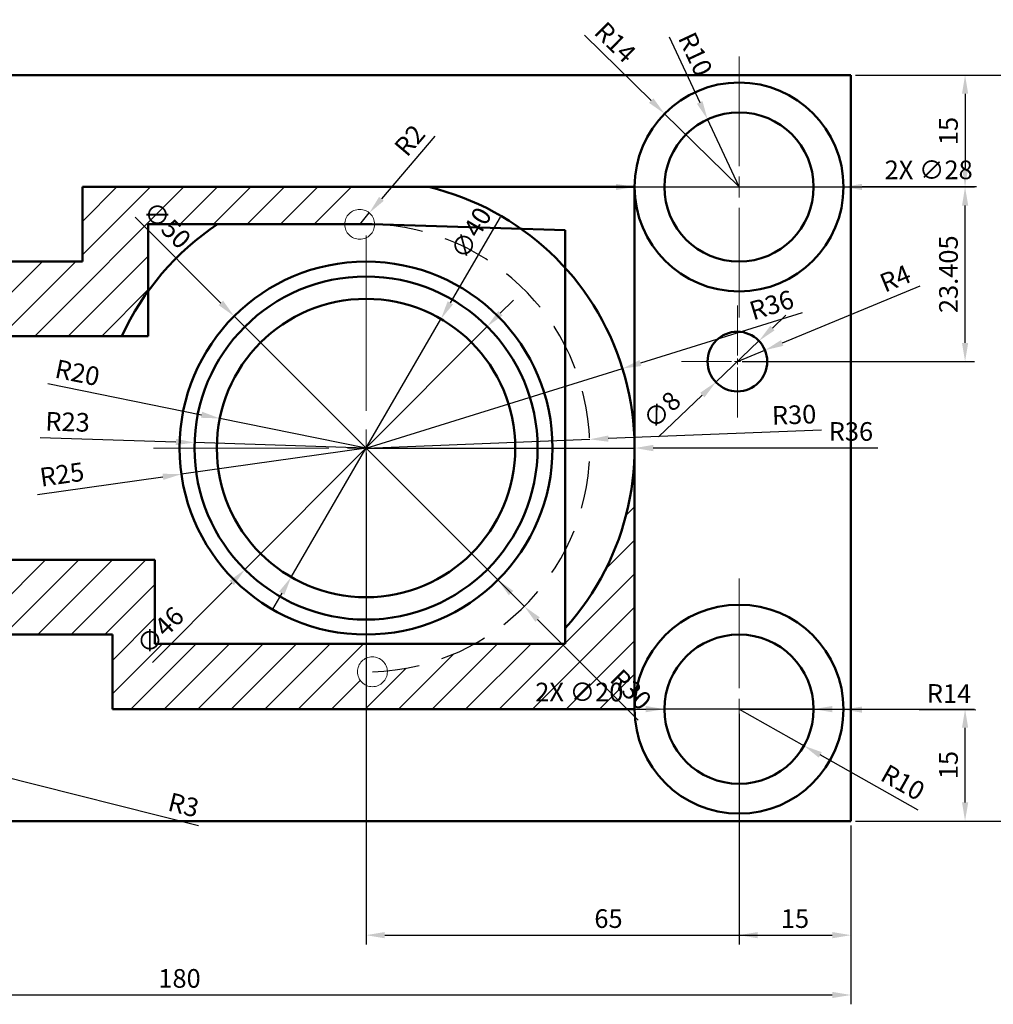
# Model space of a CAD drawing. Units: millimetres. Extents: x 1381 to 2009, y 1325 to 1613.
# Tile 2 of 6: x 1489 to 1620, y 1325 to 1457. Entities that reach past the tile are written whole.
import ezdxf

# ---------------------------------------------------------------- set-up
doc = ezdxf.new("R2010")
doc.units = ezdxf.units.MM
doc.linetypes.add('CENTER', pattern=[50.8, 31.75, -6.35, 6.35, -6.35])
doc.linetypes.add('HIDDEN', pattern=[9.525, 6.35, -3.175])
for name, color, linetype, lineweight in [('M-CNTR', 1, 'CENTER', 18), ('M-DIMS', 2, 'Continuous', 25), ('M-HATC', 8, 'Continuous', 18), ('M-HIDN', 6, 'HIDDEN', 25), ('M-OUTL', 7, 'Continuous', 50)]:
    doc.layers.add(name, color=color, linetype=linetype, lineweight=lineweight)
doc.styles.get("Standard").update_dxf_attribs({"font": 'arial.ttf'})
doc.dimstyles.new('ISO-25', dxfattribs={"dimtxt": 2.5, "dimasz": 2.5, "dimexe": 1.25, "dimexo": 0.625, "dimtad": 1, "dimtxsty": 'Standard', "dimcen": 2.5, "dimadec": 0, "dimazin": 0, "dimtfac": 1, "dimtmove": 0, "dimatfit": 3, "dimfxl": 1, "dimarcsym": 0})

# ---------------------------------------------------------------- blocks, each defined once
blk = doc.blocks.new('*U1')
blk.add_circle((0, 0), 2)
blk = doc.blocks.new('*U2')
at = {"layer": 'M-CNTR', "color": 0, "linetype": 'ByBlock', "lineweight": -2, "transparency": 16777216}
blk.add_blockref('*U1', (1534.62, 1429.72), dxfattribs=at)
at = {"layer": 'M-CNTR', "color": 0, "linetype": 'ByBlock', "lineweight": -2, "transparency": 16777216, "rotation": 180}
blk.add_blockref('*U1', (1536.33, 1369.74), dxfattribs=at)
blk = doc.blocks.new('*U6')
at = {"layer": 'M-CNTR', "color": 0, "transparency": 16777216}
for p, q in [((0, 2.8), (0, 17.5)), ((-17.5, 0), (-2.8, 0)), ((2.8, 0), (17.5, 0)), ((0, -17.5), (0, -2.8))]:
    blk.add_line(p, q, dxfattribs=at)
at = {"layer": 'M-CNTR', "color": 0, "linetype": 'Continuous', "transparency": 16777216}
for p, q in [((0, -1.4), (0, 1.4)), ((-1.4, 0), (1.4, 0))]:
    blk.add_line(p, q, dxfattribs=at)
blk = doc.blocks.new('*U7')
at = {"layer": 'M-CNTR', "color": 0, "transparency": 16777216}
for p, q in [((0, 2.8), (0, 17.5)), ((-17.5, 0), (-2.8, 0)), ((2.8, 0), (17.5, 0)), ((0, -17.5), (0, -2.8))]:
    blk.add_line(p, q, dxfattribs=at)
at = {"layer": 'M-CNTR', "color": 0, "linetype": 'Continuous', "transparency": 16777216}
for p, q in [((0, -1.4), (0, 1.4)), ((-1.4, 0), (1.4, 0))]:
    blk.add_line(p, q, dxfattribs=at)
blk = doc.blocks.new('*U8')
at = {"layer": 'M-CNTR', "color": 0, "transparency": 16777216}
for p, q in [((0, 0.8), (0, 7.5)), ((-7.5, 0), (-0.8, 0)), ((0.8, 0), (7.5, 0)), ((0, -7.5), (0, -0.8))]:
    blk.add_line(p, q, dxfattribs=at)
at = {"layer": 'M-CNTR', "color": 0, "linetype": 'Continuous', "transparency": 16777216}
for p, q in [((-0.4, 0), (0.4, 0)), ((0, -0.4), (0, 0.4))]:
    blk.add_line(p, q, dxfattribs=at)
blk = doc.blocks.new('*U9')
at = {"layer": 'M-CNTR', "color": 0, "transparency": 16777216}
for p, q in [((0, 5), (0, 28.5)), ((-28.5, 0), (-5, 0)), ((5, 0), (28.5, 0)), ((0, -28.5), (0, -5))]:
    blk.add_line(p, q, dxfattribs=at)
at = {"layer": 'M-CNTR', "color": 0, "linetype": 'Continuous', "transparency": 16777216}
for p, q in [((0, -2.5), (0, 2.5)), ((-2.5, 0), (2.5, 0))]:
    blk.add_line(p, q, dxfattribs=at)
blk = doc.blocks.new('*D38')
at = {"layer": 'Defpoints', "color": 0, "transparency": 16777216}
for p in [(1420.47, 1349.73), (1600.47, 1349.73), (1600.47, 1326.41)]:
    blk.add_point(p, dxfattribs=at)
at = {"layer": 'M-DIMS', "color": 0, "lineweight": -2, "transparency": 16777216}
for p, q in [((1420.47, 1349.11), (1420.47, 1325.16)), ((1600.47, 1349.11), (1600.47, 1325.16)), ((1422.97, 1326.41), (1597.97, 1326.41))]:
    blk.add_line(p, q, dxfattribs=at)
at = {"layer": 'M-DIMS', "color": 0, "transparency": 16777216}
for points in [[(1422.97, 1326.83), (1422.97, 1326), (1420.47, 1326.41)], [(1597.97, 1326.83), (1597.97, 1326), (1600.47, 1326.41)]]:
    blk.add_solid(points, dxfattribs=at)
at = {"layer": 'M-DIMS', "color": 0, "transparency": 16777216, "insert": (1510.47, 1328.31), "char_height": 2.5, "attachment_point": 5}
blk.add_mtext('180', dxfattribs=at)
blk = doc.blocks.new('*D39')
at = {"layer": 'Defpoints', "color": 0, "transparency": 16777216}
for p in [(1600.47, 1449.73), (1600.47, 1349.73), (1624.64, 1349.73)]:
    blk.add_point(p, dxfattribs=at)
at = {"layer": 'M-DIMS', "color": 0, "lineweight": -2, "transparency": 16777216}
for p, q in [((1601.1, 1449.73), (1625.89, 1449.73)), ((1624.64, 1447.23), (1624.64, 1352.23)), ((1601.1, 1349.73), (1625.89, 1349.73))]:
    blk.add_line(p, q, dxfattribs=at)
at = {"layer": 'M-DIMS', "color": 0, "transparency": 16777216}
for points in [[(1624.22, 1447.23), (1625.06, 1447.23), (1624.64, 1449.73)], [(1624.22, 1352.23), (1625.06, 1352.23), (1624.64, 1349.73)]]:
    blk.add_solid(points, dxfattribs=at)
at = {"layer": 'M-DIMS', "color": 0, "transparency": 16777216, "insert": (1622.74, 1399.73), "char_height": 2.5, "attachment_point": 5, "rotation": 90}
blk.add_mtext('100', dxfattribs=at)
blk = doc.blocks.new('*D41')
at = {"layer": 'Defpoints', "color": 0, "transparency": 16777216}
for p in [(1515.87, 1403.7), (1535.47, 1399.73)]:
    blk.add_point(p, dxfattribs=at)
at = {"layer": 'M-DIMS', "color": 0, "lineweight": -2, "transparency": 16777216}
for p, q in [((1492.81, 1408.37), (1513.42, 1404.2)), ((1535.47, 1399.73), (1515.87, 1403.7))]:
    blk.add_line(p, q, dxfattribs=at)
at = {"layer": 'M-DIMS', "color": 0, "transparency": 16777216}
blk.add_solid([(1513.5, 1404.6), (1513.34, 1403.79), (1515.87, 1403.7)], dxfattribs=at)
at = {"layer": 'M-DIMS', "color": 0, "transparency": 16777216, "insert": (1496.72, 1409.52), "char_height": 2.5, "attachment_point": 5, "rotation": 348.5523}
blk.add_mtext('R20', dxfattribs=at)
blk = doc.blocks.new('*D42')
at = {"layer": 'Defpoints', "color": 0, "transparency": 16777216}
for p in [(1512.48, 1400.47), (1535.47, 1399.73)]:
    blk.add_point(p, dxfattribs=at)
at = {"layer": 'M-DIMS', "color": 0, "lineweight": -2, "transparency": 16777216}
for p, q in [((1491.79, 1401.13), (1509.99, 1400.55)), ((1535.47, 1399.73), (1512.48, 1400.47))]:
    blk.add_line(p, q, dxfattribs=at)
at = {"layer": 'M-DIMS', "color": 0, "transparency": 16777216}
blk.add_solid([(1510, 1400.97), (1509.97, 1400.13), (1512.48, 1400.47)], dxfattribs=at)
at = {"layer": 'M-DIMS', "color": 0, "transparency": 16777216, "insert": (1495.46, 1402.92), "char_height": 2.5, "attachment_point": 5, "rotation": 358.1602}
blk.add_mtext('R23', dxfattribs=at)
blk = doc.blocks.new('*D43')
at = {"layer": 'Defpoints', "color": 0, "transparency": 16777216}
for p in [(1535.47, 1399.73), (1510.72, 1396.23)]:
    blk.add_point(p, dxfattribs=at)
at = {"layer": 'M-DIMS', "color": 0, "lineweight": -2, "transparency": 16777216}
for p, q in [((1535.47, 1399.73), (1510.72, 1396.23)), ((1491.43, 1393.49), (1508.24, 1395.87))]:
    blk.add_line(p, q, dxfattribs=at)
at = {"layer": 'M-DIMS', "color": 0, "transparency": 16777216}
blk.add_solid([(1508.19, 1396.29), (1508.3, 1395.46), (1510.72, 1396.23)], dxfattribs=at)
at = {"layer": 'M-DIMS', "color": 0, "transparency": 16777216, "insert": (1494.75, 1395.88), "char_height": 2.5, "attachment_point": 5, "rotation": 8.0588}
blk.add_mtext('R25', dxfattribs=at)
blk = doc.blocks.new('*D44')
at = {"layer": 'Defpoints', "color": 0, "transparency": 16777216}
for p in [(1565.45, 1400.9), (1535.47, 1399.73)]:
    blk.add_point(p, dxfattribs=at)
at = {"layer": 'M-DIMS', "color": 0, "lineweight": -2, "transparency": 16777216}
for p, q in [((1596.54, 1402.11), (1567.95, 1400.99)), ((1535.47, 1399.73), (1565.45, 1400.9))]:
    blk.add_line(p, q, dxfattribs=at)
at = {"layer": 'M-DIMS', "color": 0, "transparency": 16777216}
blk.add_solid([(1567.93, 1401.41), (1567.96, 1400.58), (1565.45, 1400.9)], dxfattribs=at)
at = {"layer": 'M-DIMS', "color": 0, "transparency": 16777216, "insert": (1592.86, 1403.87), "char_height": 2.5, "attachment_point": 5, "rotation": 2.2276}
blk.add_mtext('R30', dxfattribs=at)
blk = doc.blocks.new('*D45')
at = {"layer": 'Defpoints', "color": 0, "transparency": 16777216}
for p in [(1535.47, 1399.73), (1571.47, 1399.73)]:
    blk.add_point(p, dxfattribs=at)
at = {"layer": 'M-DIMS', "color": 0, "lineweight": -2, "transparency": 16777216}
for p, q in [((1535.47, 1399.73), (1571.47, 1399.73)), ((1604.08, 1399.73), (1573.97, 1399.73))]:
    blk.add_line(p, q, dxfattribs=at)
at = {"layer": 'M-DIMS', "color": 0, "transparency": 16777216}
blk.add_solid([(1573.97, 1400.15), (1573.97, 1399.31), (1571.47, 1399.73)], dxfattribs=at)
at = {"layer": 'M-DIMS', "color": 0, "transparency": 16777216, "insert": (1600.47, 1401.63), "char_height": 2.5, "attachment_point": 5}
blk.add_mtext('R36', dxfattribs=at)
blk = doc.blocks.new('*D46')
at = {"layer": 'Defpoints', "color": 0, "transparency": 16777216}
for p in [(1535.91, 1431.24), (1534.62, 1429.72)]:
    blk.add_point(p, dxfattribs=at)
at = {"layer": 'M-DIMS', "color": 0, "lineweight": -2, "transparency": 16777216}
for p, q in [((1544.7, 1441.55), (1537.53, 1433.14)), ((1534.62, 1429.72), (1535.91, 1431.24))]:
    blk.add_line(p, q, dxfattribs=at)
at = {"layer": 'M-DIMS', "color": 0, "transparency": 16777216}
blk.add_solid([(1537.22, 1433.41), (1537.85, 1432.87), (1535.91, 1431.24)], dxfattribs=at)
at = {"layer": 'M-DIMS', "color": 0, "transparency": 16777216, "insert": (1541.57, 1440.77), "char_height": 2.5, "attachment_point": 5, "rotation": 49.5564}
blk.add_mtext('R2', dxfattribs=at)
blk = doc.blocks.new('*D47')
at = {"layer": 'Defpoints', "color": 0, "transparency": 16777216}
for p in [(1575.49, 1444.55), (1585.47, 1434.73)]:
    blk.add_point(p, dxfattribs=at)
at = {"layer": 'M-DIMS', "color": 0, "lineweight": -2, "transparency": 16777216}
for p, q in [((1564.77, 1455.09), (1573.71, 1446.3)), ((1585.47, 1434.73), (1575.49, 1444.55))]:
    blk.add_line(p, q, dxfattribs=at)
at = {"layer": 'M-DIMS', "color": 0, "transparency": 16777216}
blk.add_solid([(1574, 1446.6), (1573.41, 1446), (1575.49, 1444.55)], dxfattribs=at)
at = {"layer": 'M-DIMS', "color": 0, "transparency": 16777216, "insert": (1568.66, 1453.9), "char_height": 2.5, "attachment_point": 5, "rotation": 315.4862}
blk.add_mtext('R14', dxfattribs=at)
blk = doc.blocks.new('*D48')
at = {"layer": 'Defpoints', "color": 0, "transparency": 16777216}
for p in [(1581.25, 1443.8), (1585.47, 1434.73)]:
    blk.add_point(p, dxfattribs=at)
at = {"layer": 'M-DIMS', "color": 0, "lineweight": -2, "transparency": 16777216}
for p, q in [((1576.1, 1454.87), (1580.2, 1446.06)), ((1585.47, 1434.73), (1581.25, 1443.8))]:
    blk.add_line(p, q, dxfattribs=at)
at = {"layer": 'M-DIMS', "color": 0, "transparency": 16777216}
blk.add_solid([(1580.57, 1446.24), (1579.82, 1445.89), (1581.25, 1443.8)], dxfattribs=at)
at = {"layer": 'M-DIMS', "color": 0, "transparency": 16777216, "insert": (1579.34, 1452.4), "char_height": 2.5, "attachment_point": 5, "rotation": 294.9613}
blk.add_mtext('R10', dxfattribs=at)
blk = doc.blocks.new('*D49')
at = {"layer": 'Defpoints', "color": 0, "transparency": 16777216}
for p in [(1588.95, 1412.85), (1585.25, 1411.33)]:
    blk.add_point(p, dxfattribs=at)
at = {"layer": 'M-DIMS', "color": 0, "lineweight": -2, "transparency": 16777216}
for p, q in [((1609.69, 1421.44), (1591.26, 1413.81)), ((1585.25, 1411.33), (1588.95, 1412.85))]:
    blk.add_line(p, q, dxfattribs=at)
at = {"layer": 'M-DIMS', "color": 0, "transparency": 16777216}
blk.add_solid([(1591.1, 1414.2), (1591.41, 1413.43), (1588.95, 1412.85)], dxfattribs=at)
at = {"layer": 'M-DIMS', "color": 0, "transparency": 16777216, "insert": (1606.54, 1422.17), "char_height": 2.5, "attachment_point": 5, "rotation": 22.4859}
blk.add_mtext('R4', dxfattribs=at)
blk = doc.blocks.new('*D50')
at = {"layer": 'Defpoints', "color": 0, "transparency": 16777216}
for p in [(1585.47, 1364.73), (1599.47, 1364.68)]:
    blk.add_point(p, dxfattribs=at)
at = {"layer": 'M-DIMS', "color": 0, "lineweight": -2, "transparency": 16777216}
for p, q in [((1585.47, 1364.73), (1599.47, 1364.68)), ((1617.22, 1364.61), (1601.97, 1364.67))]:
    blk.add_line(p, q, dxfattribs=at)
at = {"layer": 'M-DIMS', "color": 0, "transparency": 16777216}
blk.add_solid([(1601.97, 1365.08), (1601.97, 1364.25), (1599.47, 1364.68)], dxfattribs=at)
at = {"layer": 'M-DIMS', "color": 0, "transparency": 16777216, "insert": (1613.62, 1366.5), "char_height": 2.5, "attachment_point": 5, "rotation": 359.7773}
blk.add_mtext('R14', dxfattribs=at)
blk = doc.blocks.new('*D51')
at = {"layer": 'Defpoints', "color": 0, "transparency": 16777216}
for p in [(1585.47, 1364.73), (1594.18, 1359.82)]:
    blk.add_point(p, dxfattribs=at)
at = {"layer": 'M-DIMS', "color": 0, "lineweight": -2, "transparency": 16777216}
for p, q in [((1585.47, 1364.73), (1594.18, 1359.82)), ((1609.49, 1351.2), (1596.36, 1358.59))]:
    blk.add_line(p, q, dxfattribs=at)
at = {"layer": 'M-DIMS', "color": 0, "transparency": 16777216}
blk.add_solid([(1596.57, 1358.96), (1596.16, 1358.23), (1594.18, 1359.82)], dxfattribs=at)
at = {"layer": 'M-DIMS', "color": 0, "transparency": 16777216, "insert": (1607.28, 1354.63), "char_height": 2.5, "attachment_point": 5, "rotation": 330.6046}
blk.add_mtext('R10', dxfattribs=at)
blk = doc.blocks.new('*D54')
at = {"layer": 'Defpoints', "color": 0, "transparency": 16777216}
for p in [(1465.8, 1361), (1468.71, 1360.27)]:
    blk.add_point(p, dxfattribs=at)
at = {"layer": 'M-DIMS', "color": 0, "lineweight": -2, "transparency": 16777216}
for p, q in [((1465.8, 1361), (1468.71, 1360.27)), ((1513.03, 1349.08), (1471.13, 1359.66))]:
    blk.add_line(p, q, dxfattribs=at)
at = {"layer": 'M-DIMS', "color": 0, "transparency": 16777216}
blk.add_solid([(1471.23, 1360.06), (1471.03, 1359.25), (1468.71, 1360.27)], dxfattribs=at)
at = {"layer": 'M-DIMS', "color": 0, "transparency": 16777216, "insert": (1510.94, 1351.57), "char_height": 2.5, "attachment_point": 5, "rotation": 345.8378}
blk.add_mtext('R3', dxfattribs=at)
blk = doc.blocks.new('*D88')
at = {"layer": 'Defpoints', "color": 0, "transparency": 16777216}
for p in [(1535.47, 1399.73), (1600.47, 1349.73), (1600.47, 1334.43)]:
    blk.add_point(p, dxfattribs=at)
at = {"layer": 'M-DIMS', "color": 0, "lineweight": -2, "transparency": 16777216}
for p, q in [((1535.47, 1399.11), (1535.47, 1333.18)), ((1600.47, 1349.11), (1600.47, 1333.18)), ((1537.97, 1334.43), (1597.97, 1334.43))]:
    blk.add_line(p, q, dxfattribs=at)
at = {"layer": 'M-DIMS', "color": 0, "transparency": 16777216}
for points in [[(1537.97, 1334.85), (1537.97, 1334.01), (1535.47, 1334.43)], [(1597.97, 1334.85), (1597.97, 1334.01), (1600.47, 1334.43)]]:
    blk.add_solid(points, dxfattribs=at)
at = {"layer": 'M-DIMS', "color": 0, "transparency": 16777216, "insert": (1567.97, 1336.33), "char_height": 2.5, "attachment_point": 5}
blk.add_mtext('65', dxfattribs=at)
blk = doc.blocks.new('*D89')
at = {"layer": 'Defpoints', "color": 0, "transparency": 16777216}
for p in [(1585.47, 1364.73), (1615.77, 1364.73), (1600.47, 1349.73)]:
    blk.add_point(p, dxfattribs=at)
at = {"layer": 'M-DIMS', "color": 0, "lineweight": -2, "transparency": 16777216}
for p, q in [((1586.1, 1364.73), (1617.02, 1364.73)), ((1615.77, 1352.23), (1615.77, 1362.23)), ((1601.1, 1349.73), (1617.02, 1349.73))]:
    blk.add_line(p, q, dxfattribs=at)
at = {"layer": 'M-DIMS', "color": 0, "transparency": 16777216}
for points in [[(1615.36, 1362.23), (1616.19, 1362.23), (1615.77, 1364.73)], [(1615.36, 1352.23), (1616.19, 1352.23), (1615.77, 1349.73)]]:
    blk.add_solid(points, dxfattribs=at)
at = {"layer": 'M-DIMS', "color": 0, "transparency": 16777216, "insert": (1613.87, 1357.23), "char_height": 2.5, "attachment_point": 5, "rotation": 90}
blk.add_mtext('15', dxfattribs=at)
blk = doc.blocks.new('*D90')
at = {"layer": 'Defpoints', "color": 0, "transparency": 16777216}
for p in [(1600.47, 1449.73), (1585.47, 1434.73), (1615.77, 1434.73)]:
    blk.add_point(p, dxfattribs=at)
at = {"layer": 'M-DIMS', "color": 0, "lineweight": -2, "transparency": 16777216}
for p, q in [((1601.1, 1449.73), (1617.02, 1449.73)), ((1615.77, 1447.23), (1615.77, 1437.23)), ((1586.1, 1434.73), (1617.02, 1434.73))]:
    blk.add_line(p, q, dxfattribs=at)
at = {"layer": 'M-DIMS', "color": 0, "transparency": 16777216}
for points in [[(1615.36, 1447.23), (1616.19, 1447.23), (1615.77, 1449.73)], [(1615.36, 1437.23), (1616.19, 1437.23), (1615.77, 1434.73)]]:
    blk.add_solid(points, dxfattribs=at)
at = {"layer": 'M-DIMS', "color": 0, "transparency": 16777216, "insert": (1613.87, 1442.23), "char_height": 2.5, "attachment_point": 5, "rotation": 90}
blk.add_mtext('15', dxfattribs=at)
blk = doc.blocks.new('*D91')
at = {"layer": 'Defpoints', "color": 0, "transparency": 16777216}
for p in [(1585.47, 1434.73), (1615.77, 1434.73), (1585.25, 1411.33)]:
    blk.add_point(p, dxfattribs=at)
at = {"layer": 'M-DIMS', "color": 0, "lineweight": -2, "transparency": 16777216}
for p, q in [((1586.1, 1434.73), (1617.02, 1434.73)), ((1615.77, 1413.83), (1615.77, 1432.23)), ((1585.87, 1411.33), (1617.02, 1411.33))]:
    blk.add_line(p, q, dxfattribs=at)
at = {"layer": 'M-DIMS', "color": 0, "transparency": 16777216}
for points in [[(1615.36, 1432.23), (1616.19, 1432.23), (1615.77, 1434.73)], [(1615.36, 1413.83), (1616.19, 1413.83), (1615.77, 1411.33)]]:
    blk.add_solid(points, dxfattribs=at)
at = {"layer": 'M-DIMS', "color": 0, "transparency": 16777216, "insert": (1613.87, 1423.03), "char_height": 2.5, "attachment_point": 5, "rotation": 90}
blk.add_mtext('23.405', dxfattribs=at)
blk = doc.blocks.new('*D92')
at = {"layer": 'Defpoints', "color": 0, "transparency": 16777216}
for p in [(1585.47, 1364.73), (1600.47, 1349.73), (1600.47, 1334.43)]:
    blk.add_point(p, dxfattribs=at)
at = {"layer": 'M-DIMS', "color": 0, "lineweight": -2, "transparency": 16777216}
for p, q in [((1585.47, 1364.11), (1585.47, 1333.18)), ((1600.47, 1349.11), (1600.47, 1333.18)), ((1587.97, 1334.43), (1597.97, 1334.43))]:
    blk.add_line(p, q, dxfattribs=at)
at = {"layer": 'M-DIMS', "color": 0, "transparency": 16777216}
for points in [[(1587.97, 1334.85), (1587.97, 1334.01), (1585.47, 1334.43)], [(1597.97, 1334.85), (1597.97, 1334.01), (1600.47, 1334.43)]]:
    blk.add_solid(points, dxfattribs=at)
at = {"layer": 'M-DIMS', "color": 0, "transparency": 16777216, "insert": (1592.97, 1336.33), "char_height": 2.5, "attachment_point": 5}
blk.add_mtext('15', dxfattribs=at)
blk = doc.blocks.new('*D114')
at = {"layer": 'Defpoints', "color": 0, "transparency": 16777216}
for p in [(1517.79, 1417.41), (1553.15, 1382.05)]:
    blk.add_point(p, dxfattribs=at)
at = {"layer": 'M-DIMS', "color": 0, "lineweight": -2, "transparency": 16777216}
for p, q in [((1504.52, 1430.68), (1516.03, 1419.17)), ((1553.15, 1382.05), (1517.79, 1417.41)), ((1554.92, 1380.29), (1556.69, 1378.52))]:
    blk.add_line(p, q, dxfattribs=at)
at = {"layer": 'M-DIMS', "color": 0, "transparency": 16777216}
for points in [[(1516.32, 1419.47), (1515.73, 1418.88), (1517.79, 1417.41)], [(1555.21, 1380.58), (1554.62, 1379.99), (1553.15, 1382.05)]]:
    blk.add_solid(points, dxfattribs=at)
at = {"layer": 'M-DIMS', "color": 0, "transparency": 16777216, "insert": (1508.58, 1429.41), "char_height": 2.5, "attachment_point": 5, "rotation": 315.0037}
blk.add_mtext('∅50', dxfattribs=at)
blk = doc.blocks.new('*D115')
at = {"layer": 'Defpoints', "color": 0, "transparency": 16777216}
for p in [(1551.71, 1416.02), (1519.24, 1383.44)]:
    blk.add_point(p, dxfattribs=at)
at = {"layer": 'M-DIMS', "color": 0, "lineweight": -2, "transparency": 16777216}
for p, q in [((1553.47, 1417.79), (1555.24, 1419.56)), ((1551.71, 1416.02), (1519.24, 1383.44)), ((1506.83, 1370.99), (1517.47, 1381.67))]:
    blk.add_line(p, q, dxfattribs=at)
at = {"layer": 'M-DIMS', "color": 0, "transparency": 16777216}
for points in [[(1553.18, 1418.09), (1553.77, 1417.5), (1551.71, 1416.02)], [(1517.18, 1381.96), (1517.77, 1381.37), (1519.24, 1383.44)]]:
    blk.add_solid(points, dxfattribs=at)
at = {"layer": 'M-DIMS', "color": 0, "transparency": 16777216, "insert": (1508.1, 1375.05), "char_height": 2.5, "attachment_point": 5, "rotation": 45.1018}
blk.add_mtext('∅46', dxfattribs=at)
blk = doc.blocks.new('*D116')
at = {"layer": 'Defpoints', "color": 0, "transparency": 16777216}
for p in [(1545.51, 1417.03), (1525.43, 1382.43)]:
    blk.add_point(p, dxfattribs=at)
at = {"layer": 'M-DIMS', "color": 0, "lineweight": -2, "transparency": 16777216}
for p, q in [((1553.43, 1430.66), (1546.77, 1419.19)), ((1525.43, 1382.43), (1545.51, 1417.03)), ((1524.17, 1380.27), (1522.92, 1378.11))]:
    blk.add_line(p, q, dxfattribs=at)
at = {"layer": 'M-DIMS', "color": 0, "transparency": 16777216}
for points in [[(1546.41, 1419.4), (1547.13, 1418.98), (1545.51, 1417.03)], [(1523.81, 1380.48), (1524.53, 1380.06), (1525.43, 1382.43)]]:
    blk.add_solid(points, dxfattribs=at)
at = {"layer": 'M-DIMS', "color": 0, "transparency": 16777216, "insert": (1549.84, 1428.39), "char_height": 2.5, "attachment_point": 5, "rotation": 59.8582}
blk.add_mtext('∅40', dxfattribs=at)
blk = doc.blocks.new('*D117')
at = {"layer": 'Defpoints', "color": 0, "transparency": 16777216}
for p in [(1535.47, 1399.73), (1556.68, 1378.52)]:
    blk.add_point(p, dxfattribs=at)
at = {"layer": 'M-DIMS', "color": 0, "lineweight": -2, "transparency": 16777216}
for p, q in [((1535.47, 1399.73), (1556.68, 1378.52)), ((1571.96, 1363.24), (1558.45, 1376.75))]:
    blk.add_line(p, q, dxfattribs=at)
at = {"layer": 'M-DIMS', "color": 0, "transparency": 16777216}
blk.add_solid([(1558.75, 1377.04), (1558.16, 1376.45), (1556.68, 1378.52)], dxfattribs=at)
at = {"layer": 'M-DIMS', "color": 0, "transparency": 16777216, "insert": (1570.76, 1367.13), "char_height": 2.5, "attachment_point": 5, "rotation": 314.9969}
blk.add_mtext('R30', dxfattribs=at)
blk = doc.blocks.new('*D118')
at = {"layer": 'Defpoints', "color": 0, "transparency": 16777216}
for p in [(1569.86, 1410.39), (1535.47, 1399.73)]:
    blk.add_point(p, dxfattribs=at)
at = {"layer": 'M-DIMS', "color": 0, "lineweight": -2, "transparency": 16777216}
for p, q in [((1593.94, 1417.85), (1572.25, 1411.13)), ((1535.47, 1399.73), (1569.86, 1410.39))]:
    blk.add_line(p, q, dxfattribs=at)
at = {"layer": 'M-DIMS', "color": 0, "transparency": 16777216}
blk.add_solid([(1572.12, 1411.53), (1572.37, 1410.73), (1569.86, 1410.39)], dxfattribs=at)
at = {"layer": 'M-DIMS', "color": 0, "transparency": 16777216, "insert": (1589.93, 1418.6), "char_height": 2.5, "attachment_point": 5, "rotation": 17.2193}
blk.add_mtext('R36', dxfattribs=at)
blk = doc.blocks.new('*D119')
at = {"layer": 'Defpoints', "color": 0, "transparency": 16777216}
for p in [(1571.47, 1434.73), (1599.47, 1434.73)]:
    blk.add_point(p, dxfattribs=at)
at = {"layer": 'M-DIMS', "color": 0, "lineweight": -2, "transparency": 16777216}
for p, q in [((1568.97, 1434.73), (1566.47, 1434.73)), ((1571.47, 1434.73), (1599.47, 1434.73)), ((1617.31, 1434.73), (1601.97, 1434.73))]:
    blk.add_line(p, q, dxfattribs=at)
at = {"layer": 'M-DIMS', "color": 0, "transparency": 16777216}
for points in [[(1568.97, 1435.15), (1568.97, 1434.31), (1571.47, 1434.73)], [(1601.97, 1435.15), (1601.97, 1434.31), (1599.47, 1434.73)]]:
    blk.add_solid(points, dxfattribs=at)
at = {"layer": 'M-DIMS', "color": 0, "transparency": 16777216, "insert": (1610.89, 1436.7), "char_height": 2.5, "attachment_point": 5, "rotation": 359.9995}
blk.add_mtext('2X ∅28', dxfattribs=at)
blk = doc.blocks.new('*D120')
at = {"layer": 'Defpoints', "color": 0, "transparency": 16777216}
for p in [(1575.47, 1364.73), (1595.47, 1364.73)]:
    blk.add_point(p, dxfattribs=at)
at = {"layer": 'M-DIMS', "color": 0, "lineweight": -2, "transparency": 16777216}
for p, q in [((1557.65, 1364.73), (1572.97, 1364.73)), ((1595.47, 1364.73), (1575.47, 1364.73)), ((1597.97, 1364.73), (1600.47, 1364.73))]:
    blk.add_line(p, q, dxfattribs=at)
at = {"layer": 'M-DIMS', "color": 0, "transparency": 16777216}
for points in [[(1572.97, 1365.15), (1572.97, 1364.31), (1575.47, 1364.73)], [(1597.97, 1365.15), (1597.97, 1364.31), (1595.47, 1364.73)]]:
    blk.add_solid(points, dxfattribs=at)
at = {"layer": 'M-DIMS', "color": 0, "transparency": 16777216, "insert": (1564.06, 1366.7), "char_height": 2.5, "attachment_point": 5, "rotation": 0.0007}
blk.add_mtext('2X ∅20', dxfattribs=at)
blk = doc.blocks.new('*D121')
at = {"layer": 'Defpoints', "color": 0, "transparency": 16777216}
for p in [(1588.14, 1414.09), (1582.36, 1408.56)]:
    blk.add_point(p, dxfattribs=at)
at = {"layer": 'M-DIMS', "color": 0, "lineweight": -2, "transparency": 16777216}
for p, q in [((1589.95, 1415.81), (1591.76, 1417.54)), ((1588.14, 1414.09), (1582.36, 1408.56)), ((1574.68, 1401.23), (1580.55, 1406.84))]:
    blk.add_line(p, q, dxfattribs=at)
at = {"layer": 'M-DIMS', "color": 0, "transparency": 16777216}
for points in [[(1589.66, 1416.12), (1590.24, 1415.51), (1588.14, 1414.09)], [(1580.26, 1407.14), (1580.84, 1406.53), (1582.36, 1408.56)]]:
    blk.add_solid(points, dxfattribs=at)
at = {"layer": 'M-DIMS', "color": 0, "transparency": 16777216, "insert": (1575.35, 1404.6), "char_height": 2.5, "attachment_point": 5, "rotation": 43.6853}
blk.add_mtext('∅8', dxfattribs=at)

msp = doc.modelspace()

# ---------------------------------------------------------------- hatches: boundary and pattern name
at = {"layer": 'M-HATC'}
h = msp.add_hatch(dxfattribs=at)
h.set_pattern_fill('ANSI31', color=256)
h.paths.add_polyline_path([(1422.9909, 1423.1434), (1419.4301, 1423.1434), (1419.4301, 1424.7301), (1407.4722, 1424.7301), (1407.4722, 1414.7301), (1422.9909, 1414.7301)])
h.paths.add_polyline_path([(1506.2792, 1420.796), (1506.2792, 1429.7301), (1532.6154, 1429.7301, -0.40409142), (1534.5583, 1431.7171), (1534.4722, 1434.7301), (1497.4722, 1434.7301), (1497.4722, 1424.7301), (1439.9762, 1424.7301), (1439.9762, 1423.1434), (1437.9909, 1423.1434), (1437.9909, 1414.7301), (1502.746, 1414.7301, -0.04886567)])
h.paths.add_polyline_path([(1507.1646, 1384.7301), (1437.9909, 1384.7301), (1437.9909, 1376.7301), (1439.9421, 1376.7301), (1439.9401, 1374.7301), (1501.4722, 1374.7301), (1501.4722, 1364.7301), (1536.4722, 1364.7301), (1536.3861, 1367.7432, -0.42260463), (1534.329, 1369.7424, -0.40587199), (1536.2718, 1371.7415), (1536.2216, 1373.5004), (1507.1646, 1373.5004)])
h.paths.add_polyline_path([(1422.9909, 1384.7301), (1406.4722, 1384.7301), (1406.4722, 1374.7301), (1419.4301, 1374.7301), (1419.4301, 1376.7301), (1422.9909, 1376.7301)])
h.paths.add_polyline_path([(1571.4722, 1399.7301, -0.18599034), (1562.1646, 1375.5741), (1562.1646, 1373.5004), (1550.0325, 1373.5004, -0.10324325), (1538.3251, 1369.8661, -0.42401254), (1536.3861, 1367.7432), (1536.4722, 1364.7301), (1571.4722, 1364.7301)])

# ---------------------------------------------------------------- linework, layer by layer
at = {"layer": 'M-HIDN'}
msp.add_arc((1535.4722, 1399.7301), 30, 271.636577, 91.636577, dxfattribs=at)
at = {"layer": 'M-OUTL'}
for p, q in [((1420.4722, 1449.7301), (1600.4722, 1449.7301)), ((1600.4722, 1449.7301), (1585.4722, 1449.7301)), ((1600.4722, 1449.7301), (1600.4722, 1349.7301)), ((1571.4722, 1434.7301), (1497.4722, 1434.7301)), ((1497.4722, 1434.7301), (1497.4722, 1424.7301)), ((1571.4722, 1364.7301), (1571.4722, 1434.7301)), ((1506.2792, 1414.7301), (1506.2792, 1429.7301)), ((1506.2792, 1429.7301), (1536.2792, 1429.7301)), ((1562.1646, 1428.9361), (1536.2792, 1429.7301)), ((1562.1646, 1373.5004), (1562.1646, 1428.9361)), ((1497.4722, 1424.7301), (1407.4722, 1424.7301)), ((1437.9909, 1414.7301), (1506.2792, 1414.7301)), ((1437.9909, 1384.7301), (1507.1646, 1384.7301)), ((1507.1646, 1384.7301), (1507.1646, 1373.5004)), ((1501.4722, 1374.7301), (1406.4722, 1374.7301)), ((1501.4722, 1364.7301), (1501.4722, 1374.7301)), ((1507.1646, 1373.5004), (1562.1646, 1373.5004)), ((1571.4722, 1364.7301), (1501.4722, 1364.7301)), ((1600.4722, 1349.7301), (1420.4722, 1349.7301))]:
    msp.add_line(p, q, dxfattribs=at)
for centre, radius in [((1585.4722, 1434.7301), 14), ((1585.4722, 1434.7301), 10), ((1535.4722, 1399.7301), 25), ((1535.4722, 1399.7301), 23), ((1535.4722, 1399.7301), 20), ((1585.2498, 1411.3251), 4), ((1585.4722, 1364.7301), 14), ((1585.4722, 1364.7301), 10)]:
    msp.add_circle(centre, radius, dxfattribs=at)
for start, end in [(317.855707, 76.463797), (123.55731, 155.375682)]:
    msp.add_arc((1535.4722, 1399.7301), 36, start, end, dxfattribs=at)

# ---------------------------------------------------------------- block references
at = {"layer": 'M-CNTR'}
for name, p in [('*U7', (1585.4722, 1434.7301)), ('*U2', (0, 0)), ('*U9', (1535.4722, 1399.7301)), ('*U8', (1585.2498, 1411.3251)), ('*U6', (1585.4722, 1364.7301))]:
    msp.add_blockref(name, p, dxfattribs=at)

# ---------------------------------------------------------------- dimensions: what is measured, and where the dimension line sits
at = {"layer": 'M-DIMS'}
for center, mpoint, override, picture, middle in [((1585.4722, 1434.7301), (1575.489, 1444.5453), {"dimclrd": 0, "dimclre": 0, "dimclrt": 0}, '*D47', (1567.3405, 1452.5567)), ((1585.4722, 1434.7301), (1581.2521, 1443.7961), {"dimclrd": 0, "dimclre": 0, "dimclrt": 0}, '*D48', (1577.6188, 1451.6014)), ((1534.6154, 1429.7179), (1535.9128, 1431.24), {"dimclrd": 0, "dimclre": 0, "dimclrt": 0}, '*D46', (1542.9965, 1439.5505)), ((1585.2498, 1411.3251), (1588.9457, 1412.8549), {"dimclrd": 0, "dimclre": 0, "dimclrt": 0}, '*D49', (1607.2587, 1420.4351)), ((1535.4722, 1399.7301), (1569.8586, 1410.3872), {"dimdec": 0, "dimlfac": 1, "dimrnd": 0, "dimzin": 0, "dimdsep": 46, "dimlunit": 2}, '*D118', (1590.4905, 1416.7814)), ((1535.4722, 1399.7301), (1515.87, 1403.6996), {"dimclrd": 0, "dimclre": 0, "dimclrt": 0}, '*D41', (1496.3443, 1407.6536)), ((1535.4722, 1399.7301), (1512.484, 1400.4685), {"dimclrd": 0, "dimclre": 0, "dimclrt": 0}, '*D42', (1495.3955, 1401.0174)), ((1535.4722, 1399.7301), (1565.4495, 1400.8962), {"dimclrd": 0, "dimclre": 0, "dimclrt": 0}, '*D44', (1592.9377, 1401.9654)), ((1535.4722, 1399.7301), (1571.4722, 1399.7301), {"dimclrd": 0, "dimclre": 0, "dimclrt": 0}, '*D45', (1600.4722, 1399.7301)), ((1535.4722, 1399.7301), (1510.719, 1396.2254), {"dimclrd": 0, "dimclre": 0, "dimclrt": 0}, '*D43', (1495.0159, 1394.002)), ((1535.4722, 1399.7301), (1556.6842, 1378.5158), {"dimdec": 0, "dimlfac": 1, "dimrnd": 0, "dimzin": 0, "dimdsep": 46, "dimlunit": 2}, '*D117', (1569.4115, 1365.7872)), ((1585.4722, 1364.7301), (1599.4721, 1364.6757), {"dimclrd": 0, "dimclre": 0, "dimclrt": 0}, '*D50', (1613.6146, 1364.6208)), ((1585.4722, 1364.7301), (1594.1847, 1359.8218), {"dimclrd": 0, "dimclre": 0, "dimclrt": 0}, '*D51', (1606.3495, 1352.9685)), ((1465.7975, 1361.0032), (1468.7063, 1360.2692), {"dimclrd": 0, "dimclre": 0, "dimclrt": 0}, '*D54', (1510.4722, 1349.7301))]:
    dim = msp.add_radius_dim(center=center, mpoint=mpoint, dimstyle='ISO-25', override=override, dxfattribs=at)
    dim.commit()
    dim.dimension.update_dxf_attribs({"geometry": picture, "text_midpoint": middle, "dimtype": 164})
for base, p1, p2, override, picture, middle in [((1615.7722, 1434.7301), (1600.4722, 1449.7301), (1585.4722, 1434.7301), {"dimdec": 0, "dimlfac": 1, "dimrnd": 0, "dimzin": 0, "dimdsep": 46, "dimlunit": 2}, '*D90', (1613.8707, 1442.2301)), ((1624.6414, 1349.7301), (1600.4722, 1449.7301), (1600.4722, 1349.7301), {"dimclrd": 0, "dimclre": 0, "dimclrt": 0}, '*D39', (1622.74, 1399.7301)), ((1615.7722, 1434.7301), (1585.2498, 1411.3251), (1585.4722, 1434.7301), {"dimdec": 3, "dimlfac": 1, "dimrnd": 0, "dimzin": 0, "dimdsep": 46, "dimlunit": 2}, '*D91', (1613.8699, 1423.0276)), ((1615.7722, 1364.7301), (1600.4722, 1349.7301), (1585.4722, 1364.7301), {"dimdec": 0, "dimlfac": 1, "dimrnd": 0, "dimzin": 0, "dimdsep": 46, "dimlunit": 2}, '*D89', (1613.8707, 1357.2301))]:
    dim = msp.add_linear_dim(base=base, p1=p1, p2=p2, angle=90, dimstyle='ISO-25', override=override, dxfattribs=at)
    dim.commit()
    dim.dimension.update_dxf_attribs({"geometry": picture, "text_midpoint": middle})
dim = msp.add_diameter_dim_2p(p1=(1571.4722, 1434.7302), p2=(1599.4722, 1434.73), text='2X <>', dimstyle='ISO-25', override={"dimdec": 0, "dimlfac": 1, "dimrnd": 0, "dimzin": 0, "dimdsep": 46, "dimlunit": 2}, dxfattribs=at)
dim.commit()
dim.dimension.update_dxf_attribs({"geometry": '*D119', "text_midpoint": (1610.891, 1434.7299)})
for p1, p2, picture, middle in [((1553.151, 1382.0536), (1517.7934, 1417.4066), '*D114', (1507.1861, 1428.0126)), ((1525.4293, 1382.4344), (1545.515, 1417.0258), '*D116', (1551.5407, 1427.4033)), ((1551.7067, 1416.0225), (1519.2376, 1383.4378), '*D115', (1509.4969, 1373.6624)), ((1588.1424, 1414.0879), (1582.3572, 1408.5623), '*D121', (1576.7117, 1403.17))]:
    dim = msp.add_diameter_dim_2p(p1=p1, p2=p2, dimstyle='ISO-25', override={"dimdec": 0, "dimlfac": 1, "dimrnd": 0, "dimzin": 0, "dimdsep": 46, "dimlunit": 2}, dxfattribs=at)
    dim.commit()
    dim.dimension.update_dxf_attribs({"geometry": picture, "text_midpoint": middle, "dimtype": 163})
for base, p1, override, picture, middle in [((1600.4722, 1334.4301), (1535.4722, 1399.7301), {"dimdec": 0, "dimlfac": 1, "dimrnd": 0, "dimzin": 0, "dimdsep": 46, "dimlunit": 2}, '*D88', (1567.9722, 1336.3316)), ((1600.4722, 1334.4301), (1585.4722, 1364.7301), {"dimdec": 0, "dimlfac": 1, "dimrnd": 0, "dimzin": 0, "dimdsep": 46, "dimlunit": 2}, '*D92', (1592.9722, 1336.3316)), ((1600.4722, 1326.4121), (1420.4722, 1349.7301), {"dimclrd": 0, "dimclre": 0, "dimclrt": 0}, '*D38', (1510.4722, 1328.3136))]:
    dim = msp.add_linear_dim(base=base, p1=p1, p2=(1600.4722, 1349.7301), dimstyle='ISO-25', override=override, dxfattribs=at)
    dim.commit()
    dim.dimension.update_dxf_attribs({"geometry": picture, "text_midpoint": middle})
dim = msp.add_diameter_dim_2p(p1=(1595.4722, 1364.7302), p2=(1575.4722, 1364.73), text='2X <>', dimstyle='ISO-25', override={"dimdec": 0, "dimlfac": 1, "dimrnd": 0, "dimzin": 0, "dimdsep": 46, "dimlunit": 2}, dxfattribs=at)
dim.commit()
dim.dimension.update_dxf_attribs({"geometry": '*D120', "text_midpoint": (1564.0602, 1364.7299), "dimtype": 163})

doc.saveas('drawing.dxf')
